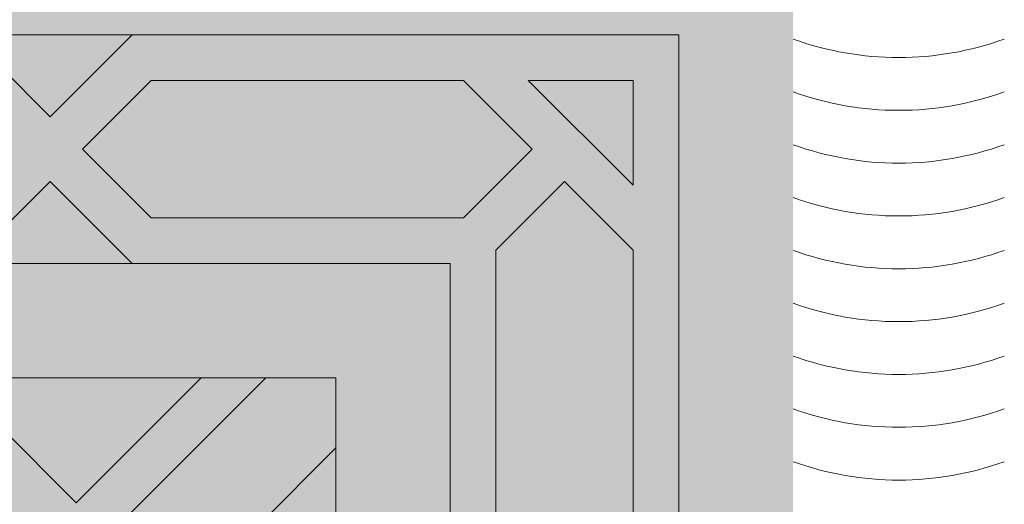
# Model space of a CAD drawing. Units: inches. Extents: x 844 to 2234, y 346 to 1084.
# Tile 39 of 93: x 1260.074 to 1265.567, y 705.079 to 707.782. Entities that reach past the tile are written whole.
import ezdxf

# ---------------------------------------------------------------- set-up
doc = ezdxf.new("R2010")
doc.units = ezdxf.units.IN
doc.header["$MEASUREMENT"] = 0
doc.layers.add('furniture', color=8, linetype='Continuous', lineweight=18)
doc.layers.add('RA-AP-01$0$INT', color=35, linetype='Continuous', lineweight=5)
doc.layers.add('RA-AP-01$0$FURN', color=3, linetype='Continuous')

# ---------------------------------------------------------------- blocks, each defined once
blk = doc.blocks.new('A$C18D01794')
at = {"layer": 'RA-AP-01$0$INT'}
h = blk.add_hatch(color=256, dxfattribs=at)
h.paths.add_polyline_path([(4.355206456958071, -6.156712009588037), (4.355206456958071, -8.056712009588038), (5.455206456958072, -8.056712009588038), (5.455206456958072, -6.156712009588037)])
h.paths.add_polyline_path([(4.405206456958072, -8.006712009588039), (4.405206456958072, -6.206712009588038), (5.405206456958072, -6.206712009588038), (5.405206456958072, -8.006712009588039)], flags=16)
h = blk.add_hatch(color=256, dxfattribs=at)
h.paths.add_polyline_path([(4.505206456958071, -7.585498806127123), (4.46934859260189, -7.549640941759413), (4.505206456958071, -7.513783077414768), (4.505206456958071, -7.381963272220687), (4.469348592616735, -7.346105407867824), (4.505206456958071, -7.310247543514964), (4.505206456958071, -7.178427738324996), (4.469348592586679, -7.142569873965138), (4.505206456952245, -7.106712009588038), (4.476922185709333, -7.106712009588038), (4.455206456960671, -7.128427738343681), (4.433490728198047, -7.106712009588038), (4.405206456946033, -7.106712009588036), (4.441064321339216, -7.142569873969684), (4.40520645695807, -7.178427738362358), (4.405206456958072, -7.310247543472698), (4.441064321364728, -7.346105407867826), (4.40520645695807, -7.381963272262947), (4.40520645695807, -7.513783077378263), (4.441064321354429, -7.549640941786153), (4.405206456958072, -7.585498806170974), (4.405206456958072, -7.717318611286652), (4.441064321333084, -7.753176475673194), (4.405206456958072, -7.789034340036673), (4.405206456958072, -8.006712009588039), (4.644348592588106, -8.006712009588039), (4.680206456964639, -7.970854145211967), (4.716064321341165, -8.006712009588039), (4.869348592586113, -8.006712009588039), (4.905206456964143, -7.970854145210465), (4.941064321342174, -8.006712009588039), (5.094348592587118, -8.006712009588037), (5.130206456963649, -7.970854145211967), (5.166064321340178, -8.006712009588039), (5.405206456958072, -8.006712009588039), (5.405206456958072, -7.789034340024526), (5.369348592595202, -7.753176475673196), (5.40520645695807, -7.717318611298797), (5.40520645695807, -7.585498806158829), (5.369348592573859, -7.549640941786151), (5.40520645695807, -7.51378307739041), (5.40520645695807, -7.381963272250803), (5.36934859256356, -7.346105407867824), (5.405206456958072, -7.310247543484846), (5.405206456958072, -7.178427738350217), (5.369348592589068, -7.142569873969682), (5.405206456982249, -7.106712009588038), (5.376922185730244, -7.106712009588038), (5.355206456967613, -7.128427738343679), (5.333490728218955, -7.10671200958804), (5.305206456976043, -7.106712009588042), (5.341064321341609, -7.142569873965136), (5.305206456958072, -7.178427738337141), (5.305206456958072, -7.310247543502816), (5.34106432131155, -7.346105407867824), (5.305206456958072, -7.381963272232832), (5.30520645695807, -7.513783077402624), (5.341064321326395, -7.549640941759413), (5.305206456958072, -7.585498806139263), (5.305206456958072, -7.717318611299605), (5.341064321347738, -7.753176475677737), (5.305206456958072, -7.78903434007894), (5.30520645695807, -7.906712009588039), (5.166064321336834, -7.906712009588039), (5.130206456963647, -7.942569873961684), (5.094348592590464, -7.906712009588039), (4.941064321338827, -7.906712009588041), (4.905206456964145, -7.942569873963183), (4.869348592589459, -7.906712009588039), (4.716064321337822, -7.906712009588041), (4.680206456964641, -7.942569873961684), (4.644348592591453, -7.906712009588039), (4.505206456958071, -7.906712009588039), (4.505206456958071, -7.789034340066795), (4.469348592580545, -7.753176475677738), (4.505206456958071, -7.717318611311748)])
h.paths.add_polyline_path([(4.485206456974132, -7.709034340046354), (4.45520645695909, -7.739034340051736), (4.425206456974128, -7.709034340057131), (4.425206456993394, -7.593783077384998), (4.45520645699153, -7.563783077396511), (4.485206456993396, -7.593783077408017)], flags=16)
h.paths.add_polyline_path([(4.455206456954537, -7.767318611299197), (4.485206456958242, -7.797318611312542), (4.48520645695951, -7.912569873958716), (4.45520645695415, -7.942569873954422), (4.425206456957888, -7.912569873967813), (4.425206456957888, -7.797318611286197)], flags=16)
h.paths.add_polyline_path([(4.455206456964794, -7.535498806149051), (4.42520645696469, -7.5054988061393), (4.425206456983954, -7.390247543486406), (4.455206456990734, -7.360247543489279), (4.485206456983953, -7.39024754349214), (4.485206456964687, -7.505498806158811)], flags=16)
h.paths.add_polyline_path([(4.499348592588947, -7.926712009585049), (4.636064321340932, -7.926712009585049), (4.666064321342317, -7.956712009586821), (4.636064321343707, -7.986712009585048), (4.499348592575121, -7.986712009585048), (4.469348592591685, -7.956712009591957)], flags=16)
h.paths.add_polyline_path([(4.425206456957888, -7.940854145195974), (4.471064321332215, -7.986712009585049), (4.425206456957888, -7.986712009585049)], flags=16)
h.paths.add_polyline_path([(4.455206456990734, -7.331963272246367), (4.425206456989053, -7.301963272254337), (4.425206456969784, -7.186712009596224), (4.455206456965226, -7.156712009591144), (4.485206456969787, -7.186712009586051), (4.485206456989053, -7.301963272238404)], flags=16)
h.paths.add_polyline_path([(4.72434859258714, -7.926712009586255), (4.861064321340141, -7.926712009586248), (4.891064321340324, -7.956712009586823), (4.861064321340513, -7.986712009586252), (4.724348592586768, -7.986712009586252), (4.694348592586956, -7.956712009586821)], flags=16)
h.paths.add_polyline_path([(4.919348592587961, -7.956712009586821), (4.949348592588145, -7.92671200958625), (5.08606432134115, -7.926712009586253), (5.116064321341327, -7.956712009586823), (5.086064321341519, -7.986712009586252), (4.949348592587774, -7.986712009586252)], flags=16)
h.paths.add_polyline_path([(5.144348592585967, -7.956712009586823), (5.174348592587358, -7.926712009585049), (5.311064321339338, -7.926712009585049), (5.3410643213366, -7.956712009591957), (5.311064321353163, -7.986712009585048), (5.174348592584576, -7.986712009585048)], flags=16)
h.paths.add_polyline_path([(5.32520645693489, -7.593783077408021), (5.355206456936755, -7.563783077396511), (5.385206456934894, -7.593783077384998), (5.38520645695416, -7.709034340057128), (5.355206456969194, -7.739034340051736), (5.325206456954153, -7.709034340046352)], flags=16)
h.paths.add_polyline_path([(5.325206456970042, -7.797318611312542), (5.355206456973747, -7.767318611299197), (5.385206456970398, -7.7973186112862), (5.385206456970398, -7.912569873967816), (5.355206456974136, -7.942569873954422), (5.325206456968778, -7.912569873958716)], flags=16)
h.paths.add_polyline_path([(5.325206456963599, -7.505498806158811), (5.325206456944333, -7.39024754349214), (5.355206456937552, -7.360247543489279), (5.385206456944332, -7.39024754348641), (5.385206456963596, -7.505498806139303), (5.355206456963492, -7.53549880614905)], flags=16)
h.paths.add_polyline_path([(5.32520645693923, -7.301963272238403), (5.3252064569585, -7.186712009586051), (5.355206456963062, -7.156712009591142), (5.3852064569585, -7.186712009596224), (5.385206456939234, -7.301963272254338), (5.355206456937552, -7.331963272246369)], flags=16)
h.paths.add_polyline_path([(5.339348592596071, -7.986712009585048), (5.385206456970398, -7.940854145195972), (5.385206456970396, -7.986712009585048)], flags=16)
h = blk.add_hatch(color=256, dxfattribs=at)
h.paths.add_polyline_path([(4.469348592586677, -7.142569873965136), (4.505206456958073, -7.178427738324996), (4.505206456958071, -7.106712009582215)])
h.paths.add_polyline_path([(4.455206456960671, -7.128427738343681), (4.476922185709333, -7.106712009588038), (4.433490728198045, -7.106712009588038)])
h.paths.add_polyline_path([(4.405206456958073, -7.178427738362358), (4.441064321339218, -7.142569873969684), (4.40520645695807, -7.106712009600073)])
h.paths.add_polyline_path([(4.425206456989053, -7.301963272254335), (4.455206456990736, -7.331963272246371), (4.485206456989055, -7.301963272238399), (4.48520645696979, -7.186712009586054), (4.455206456965227, -7.15671200959114), (4.425206456969784, -7.186712009596224)])
h.paths.add_polyline_path([(4.505206456958073, -7.381963272220689), (4.505206456958071, -7.310247543514961), (4.469348592616738, -7.346105407867826)])
h.paths.add_polyline_path([(4.425206456964688, -7.5054988061393), (4.455206456964794, -7.535498806149051), (4.485206456964689, -7.505498806158811), (4.485206456983951, -7.390247543492138), (4.455206456990736, -7.360247543489277), (4.425206456983956, -7.39024754348641)])
h.paths.add_polyline_path([(4.425206456974126, -7.709034340057128), (4.455206456959092, -7.739034340051736), (4.485206456974132, -7.709034340046356), (4.485206456993396, -7.593783077408017), (4.45520645699153, -7.563783077396511), (4.425206456993394, -7.593783077384999)])
h.paths.add_polyline_path([(4.46934859260189, -7.549640941759415), (4.505206456958071, -7.585498806127123), (4.505206456958073, -7.513783077414766)])
h.paths.add_polyline_path([(4.405206456958073, -7.585498806170972), (4.441064321354427, -7.549640941786151), (4.405206456958072, -7.513783077378263)])
h.paths.add_polyline_path([(4.405206456958072, -7.789034340036673), (4.441064321333084, -7.753176475673194), (4.405206456958072, -7.71731861128665)])
h.paths.add_polyline_path([(4.469348592580547, -7.75317647567774), (4.505206456958071, -7.789034340066795), (4.505206456958071, -7.717318611311744)])
h.paths.add_polyline_path([(4.425206456957888, -7.912569873967814), (4.45520645695415, -7.942569873954422), (4.485206456959507, -7.912569873958718), (4.48520645695824, -7.797318611312542), (4.455206456954537, -7.767318611299197), (4.425206456957888, -7.797318611286202)])
h.paths.add_polyline_path([(4.425206456957888, -7.986712009585049), (4.471064321332215, -7.986712009585049), (4.425206456957888, -7.940854145195972)])
h.paths.add_polyline_path([(4.499348592575121, -7.986712009585048), (4.636064321343707, -7.986712009585049), (4.666064321342317, -7.956712009586823), (4.636064321340932, -7.926712009585049), (4.499348592588945, -7.926712009585049), (4.469348592591685, -7.95671200959196)])
h.paths.add_polyline_path([(4.680206456964641, -7.942569873961684), (4.716064321337824, -7.906712009588039), (4.644348592591454, -7.906712009588039)])
h.paths.add_polyline_path([(4.644348592588108, -8.006712009588039), (4.716064321341167, -8.006712009588039), (4.680206456964637, -7.970854145211964)])
h.paths.add_polyline_path([(4.724348592586768, -7.98671200958625), (4.861064321340514, -7.986712009586252), (4.891064321340324, -7.956712009586819), (4.861064321340141, -7.92671200958625), (4.724348592587134, -7.926712009586255), (4.694348592586957, -7.956712009586821)])
h.paths.add_polyline_path([(4.905206456964143, -7.942569873963183), (4.941064321338827, -7.906712009588039), (4.869348592589457, -7.906712009588037)])
h.paths.add_polyline_path([(4.869348592586113, -8.006712009588039), (4.941064321342172, -8.006712009588037), (4.905206456964145, -7.970854145210463)])
h.paths.add_polyline_path([(4.949348592587774, -7.986712009586252), (5.086064321341521, -7.986712009586252), (5.116064321341329, -7.956712009586823), (5.08606432134115, -7.926712009586253), (4.949348592588145, -7.92671200958625), (4.919348592587961, -7.956712009586819)])
h.paths.add_polyline_path([(5.130206456963645, -7.942569873961684), (5.166064321336834, -7.906712009588039), (5.094348592590464, -7.906712009588039)])
h.paths.add_polyline_path([(5.094348592587119, -8.006712009588039), (5.166064321340178, -8.006712009588039), (5.130206456963651, -7.970854145211967)])
h.paths.add_polyline_path([(5.174348592584578, -7.986712009585048), (5.311064321353163, -7.986712009585048), (5.341064321336602, -7.956712009591958), (5.31106432133934, -7.926712009585049), (5.174348592587352, -7.926712009585049), (5.144348592585969, -7.956712009586823)])
h.paths.add_polyline_path([(5.325206456968778, -7.912569873958718), (5.355206456974136, -7.942569873954422), (5.385206456970396, -7.912569873967814), (5.385206456970396, -7.797318611286199), (5.355206456973747, -7.767318611299197), (5.325206456970044, -7.797318611312544)])
h.paths.add_polyline_path([(5.339348592596073, -7.986712009585048), (5.385206456970396, -7.986712009585049), (5.385206456970398, -7.94085414519597)])
h.paths.add_polyline_path([(5.325206456954155, -7.709034340046354), (5.355206456969194, -7.739034340051734), (5.38520645695416, -7.709034340057128), (5.385206456934896, -7.593783077384999), (5.355206456936758, -7.563783077396513), (5.325206456934888, -7.593783077408019)])
h.paths.add_polyline_path([(5.305206456958072, -7.789034340078938), (5.341064321347739, -7.753176475677738), (5.305206456958072, -7.717318611299605)])
h.paths.add_polyline_path([(5.369348592595204, -7.753176475673194), (5.40520645695807, -7.789034340024526), (5.405206456958072, -7.717318611298798)])
h.paths.add_polyline_path([(5.405206456958072, -7.585498806158831), (5.405206456958072, -7.513783077390407), (5.369348592573857, -7.549640941786151)])
h.paths.add_polyline_path([(5.305206456958072, -7.585498806139266), (5.341064321326393, -7.549640941759413), (5.305206456958072, -7.513783077402626)])
h.paths.add_polyline_path([(5.325206456963599, -7.50549880615881), (5.355206456963494, -7.535498806149055), (5.385206456963598, -7.505498806139302), (5.385206456944334, -7.390247543486411), (5.355206456937552, -7.360247543489279), (5.325206456944333, -7.39024754349214)])
h.paths.add_polyline_path([(5.305206456958072, -7.38196327223283), (5.341064321311551, -7.346105407867824), (5.305206456958072, -7.31024754350282)])
h.paths.add_polyline_path([(5.325206456939231, -7.301963272238404), (5.355206456937552, -7.331963272246369), (5.385206456939235, -7.301963272254335), (5.385206456958502, -7.186712009596224), (5.355206456963061, -7.156712009591142), (5.3252064569585, -7.186712009586051)])
h.paths.add_polyline_path([(5.404581768715993, -7.381338584008926, -0.001217816984214), (5.405206456958072, -7.381112009582329), (5.405206456958072, -7.310247543484846), (5.369348592563558, -7.346105407867826)])
h.paths.add_polyline_path([(5.36934859258907, -7.142569873969684), (5.40520645695807, -7.178427738350215), (5.405206456958072, -7.106712009612218)])
h.paths.add_polyline_path([(5.355206456967613, -7.128427738343683), (5.376922185730239, -7.106712009588038), (5.333490728218953, -7.10671200958804)])
h.paths.add_polyline_path([(5.30520645695807, -7.178427738337139), (5.341064321341609, -7.142569873965134), (5.305206456958074, -7.10671200957007)])
blk.add_hatch(color=256, dxfattribs=at).paths.add_polyline_path([(4.505206456958071, -7.906712009588039), (5.305206456958072, -7.906712009588039), (5.305206456958072, -7.106712009588038), (5.255206456951893, -7.106712009588036), (5.25520645694868, -7.856712009570104), (4.555206456959269, -7.856712009588616), (4.555206456956052, -7.106712009588038), (4.505206456958073, -7.106712009588038)])
h = blk.add_hatch(color=256, dxfattribs=at)
h.paths.add_polyline_path([(4.585917135068448, -7.856712009587804), (4.614201406330596, -7.856712009587056), (4.668846067270487, -7.802067348644738), (4.723490728212344, -7.856712009584164), (4.771774999457151, -7.856712009582887), (4.826419660396886, -7.80206734864072), (4.862780050090322, -7.838427738332541), (4.844495778842715, -7.856712009580965), (4.862780050090411, -7.856712009580482), (4.905206456960182, -7.814285602707865), (4.947632863832445, -7.856712009578238), (4.965917135079675, -7.856712009577755), (4.947632863831759, -7.838427738330656), (4.983993253523576, -7.802067348637219), (5.038637914464627, -7.856712009575829), (5.08692218571208, -7.856712009574554), (5.141566846649976, -7.802067348634224), (5.196211507589851, -7.856712009571666), (5.224495778822615, -7.856712009570916), (4.905206456953975, -7.537422687702283)])
h.paths.add_polyline_path([(4.895206456956031, -7.575706958950402), (4.895206456958921, -7.684996280828174), (4.840561796018589, -7.630351619890275)], flags=16)
h.paths.add_polyline_path([(4.915206456955638, -7.575706958949956), (4.969851117895509, -7.630351619887399), (4.915206456957609, -7.684996280827732)], flags=16)
h.paths.add_polyline_path([(4.826419660395175, -7.644493755514321), (4.881064321335613, -7.699138416452331), (4.771774999456703, -7.69913841645522)], flags=16)
h.paths.add_polyline_path([(4.983993253519558, -7.644493755510815), (5.038637914460456, -7.699138416449285), (4.929348592581548, -7.69913841645126)], flags=16)
h.paths.add_polyline_path([(4.881064321336025, -7.719138416452334), (4.826419660397532, -7.773783077393256), (4.771774999457062, -7.719138416455217)], flags=16)
h.paths.add_polyline_path([(4.929348592582019, -7.71913841645126), (5.038637914460982, -7.719138416449284), (4.983993253522945, -7.773783077389749)], flags=16)
h.paths.add_polyline_path([(4.895206456960191, -7.733280552075633), (4.895206456962115, -7.806001331460164), (4.876922185715016, -7.824285602708492), (4.840561796021581, -7.787925213016675)], flags=16)
h.paths.add_polyline_path([(4.915206456958487, -7.733280552075187), (4.969851117899527, -7.787925213013798), (4.933490728206909, -7.824285602708034), (4.9152064569598, -7.806001331461736)], flags=16)
h.paths.add_polyline_path([(4.757632863832376, -7.733280552079264), (4.812277524772842, -7.787925213017304), (4.757632863834348, -7.842569873958233)], flags=16)
h.paths.add_polyline_path([(4.737632863832376, -7.73328055207979), (4.737632863834348, -7.842569873958701), (4.682988202893906, -7.787925213020692)], flags=16)
h.paths.add_polyline_path([(5.05278005008503, -7.733280552072701), (5.052780050087917, -7.842569873951664), (4.998135389146995, -7.787925213013169)], flags=16)
h.paths.add_polyline_path([(5.072780050085024, -7.733280552072333), (5.127424711025931, -7.787925213010806), (5.072780050087916, -7.842569873951244)], flags=16)
h.paths.add_polyline_path([(4.935917135072783, -7.506712009583784), (5.255206456948811, -7.826001331459767), (5.255206456948932, -7.797717060211899), (5.200561796010279, -7.743072399273238), (5.255206456949403, -7.688427738334128), (5.25520645694961, -7.640143467086677), (5.200561796009787, -7.585498806146837), (5.236922185702417, -7.549138416454212), (5.255206456949919, -7.56742268770172), (5.255206456949998, -7.549138416454178), (5.212780050078687, -7.506712009583814), (5.25520645695036, -7.464285602712145), (5.255206456950438, -7.446001331464763), (5.236922185702424, -7.464285602712779), (5.200561796009796, -7.427925213020149), (5.255206456950753, -7.373280552079203), (5.25520645695096, -7.324996280834394), (5.200561796010322, -7.270351619893748), (5.255206456951428, -7.215706958952649), (5.255206456951547, -7.187422687705071)])
h.paths.add_polyline_path([(5.042988202883395, -7.42792521302065), (5.097632863823085, -7.373280552080975), (5.097632863822622, -7.482569873959883)], flags=16)
h.paths.add_polyline_path([(5.028846067259663, -7.442067348644384), (5.083490728198774, -7.496712009583504), (4.974201406321001, -7.496712009583035)], flags=16)
h.paths.add_polyline_path([(5.117632863823087, -7.37328055208089), (5.172277524762331, -7.42792521302015), (5.11763286382262, -7.482569873959851)], flags=16)
h.paths.add_polyline_path([(5.08349072819877, -7.516712009582191), (5.028846067259652, -7.571356670521302), (4.974201406320998, -7.516712009582638)], flags=16)
h.paths.add_polyline_path([(5.131774999446817, -7.35913841645716), (5.186419660386065, -7.413783077396415), (5.241064321325782, -7.359138416456712)], flags=17)
h.paths.add_polyline_path([(5.131774999446228, -7.496712009583703), (5.186419660386065, -7.442067348643883), (5.222780050079488, -7.478427738337313), (5.204495778832781, -7.496712009584014)], flags=16)
h.paths.add_polyline_path([(5.097632863822613, -7.530854145205813), (5.097632863823061, -7.640143467084723), (5.042988202883383, -7.585498806145032)], flags=16)
h.paths.add_polyline_path([(5.131774999446899, -7.339138416457162), (5.241064321325809, -7.339138416456712), (5.186419660386591, -7.284493755517479)], flags=17)
h.paths.add_polyline_path([(5.131774999446226, -7.516712009581999), (5.204495778830767, -7.516712009581702), (5.22278005007868, -7.534996280829206), (5.186419660386049, -7.571356670521828)], flags=16)
h.paths.add_polyline_path([(5.11763286382262, -7.530854145205852), (5.17227752476232, -7.585498806145562), (5.117632863823064, -7.64014346708481)], flags=16)
h.paths.add_polyline_path([(5.186419660386069, -7.599640941770585), (5.241064321325754, -7.654285602710281), (5.131774999446791, -7.654285602709814)], flags=16)
h.paths.add_polyline_path([(5.131774999446872, -7.674285602709813), (5.24106432132578, -7.674285602710282), (5.186419660386554, -7.728930263649504)], flags=16)
h.paths.add_polyline_path([(5.255206456951811, -7.126001331467467), (5.255206456951895, -7.106712009588038), (4.555206456956052, -7.106712009588038), (4.555206456956136, -7.12600133146746), (4.905206456953973, -7.476001331465289)])
h.paths.add_polyline_path([(4.983993253513404, -7.368930263651977), (4.92934859257295, -7.314285602713969), (5.03863791445186, -7.314285602711063)], flags=16)
h.paths.add_polyline_path([(4.969851117889988, -7.383072399276016), (4.915206456952556, -7.437717060215906), (4.915206456949648, -7.328427738338133)], flags=16)
h.paths.add_polyline_path([(4.929348592572535, -7.294285602713971), (4.983993253511019, -7.239640941773039), (5.038637914451496, -7.294285602711065)], flags=16)
h.paths.add_polyline_path([(5.052780050074912, -7.280143467087016), (4.998135389134438, -7.225498806148989), (5.052780050072919, -7.170854145208052)], flags=16)
h.paths.add_polyline_path([(5.07278005007491, -7.280143467086489), (5.072780050072918, -7.170854145207579), (5.127424711013374, -7.225498806145578)], flags=16)
h.paths.add_polyline_path([(4.89520645695295, -7.437717060216355), (4.840561796013067, -7.383072399278919), (4.895206456950961, -7.328427738338582)], flags=16)
h.paths.add_polyline_path([(4.915206456948365, -7.280143467090674), (4.915206456946434, -7.207422687704125), (4.933490728192729, -7.18913841645701), (4.969851117886972, -7.225498806149623)], flags=16)
h.paths.add_polyline_path([(4.881064321327021, -7.314285602715054), (4.82641966038902, -7.368930263655506), (4.771774999448108, -7.314285602717047)], flags=16)
h.paths.add_polyline_path([(4.895206456950073, -7.280143467091125), (4.840561796009022, -7.225498806152518), (4.876922185700835, -7.18913841645908), (4.895206456948749, -7.207422687706589)], flags=16)
h.paths.add_polyline_path([(4.983993253510392, -7.211356670525576), (4.947632863816944, -7.174996280833758), (4.965917135064043, -7.156712009585847), (5.038637914448995, -7.156712009584522)], flags=16)
h.paths.add_polyline_path([(4.881064321326543, -7.294285602715056), (4.771774999447578, -7.294285602717046), (4.826419660385607, -7.239640941776569)], flags=16)
h.paths.add_polyline_path([(4.905206456946447, -7.19913841645844), (4.862780050074785, -7.156712009587725), (4.947632863816685, -7.156712009586302)], flags=16)
h.paths.add_polyline_path([(5.14156684663679, -7.211356670521528), (5.086922185696452, -7.156712009583639), (5.196211507574223, -7.156712009581651)], flags=16)
h.paths.add_polyline_path([(4.8264196603837, -7.211356670529104), (4.771774999442643, -7.156712009590501), (4.8444957788276, -7.156712009588568), (4.862780050075511, -7.17499628083566)], flags=16)
h.paths.add_polyline_path([(4.812277524760289, -7.225498806153156), (4.757632863822258, -7.28014346709363), (4.757632863819352, -7.170854145214669)], flags=16)
h.paths.add_polyline_path([(4.73763286382226, -7.280143467093997), (4.682988202881349, -7.22549880615554), (4.737632863819352, -7.170854145215086)], flags=16)
h.paths.add_polyline_path([(4.723490728195188, -7.156712009591787), (4.668846067257299, -7.211356670532127), (4.614201406317417, -7.156712009594693)], flags=16)
h.paths.add_polyline_path([(4.597632863829262, -7.506712009583814), (4.555206456957951, -7.54913841645418), (4.555206456958029, -7.56742268770172), (4.573490728205535, -7.549138416454212), (4.609851117898167, -7.585498806146839), (4.555206456958338, -7.640143467086675), (4.555206456958546, -7.688427738334125), (4.60985111789767, -7.743072399273238), (4.555206456959015, -7.797717060211899), (4.555206456959138, -7.826001331459767), (4.874495778835167, -7.506712009583786), (4.5552064569564, -7.187422687705062), (4.555206456956523, -7.215706958952644), (4.609851117897629, -7.270351619893746), (4.555206456956988, -7.324996280834396), (4.555206456957198, -7.373280552079195), (4.609851117898153, -7.427925213020147), (4.573490728205528, -7.464285602712779), (4.555206456957507, -7.446001331464756), (4.555206456957585, -7.464285602712143)])
h.paths.add_polyline_path([(4.712780050085332, -7.482569873959882), (4.712780050084863, -7.373280552080972), (4.767424711024555, -7.42792521302065)], flags=16)
h.paths.add_polyline_path([(4.726922185709173, -7.496712009583504), (4.781566846648288, -7.442067348644384), (4.836211507586949, -7.496712009583033)], flags=16)
h.paths.add_polyline_path([(4.692780050085327, -7.482569873959851), (4.638135389145619, -7.427925213020149), (4.692780050084865, -7.373280552080892)], flags=16)
h.paths.add_polyline_path([(4.726922185709182, -7.516712009582191), (4.836211507586949, -7.51671200958264), (4.7815668466483, -7.571356670521304)], flags=16)
h.paths.add_polyline_path([(4.678637914461726, -7.496712009583706), (4.605917135075169, -7.496712009584014), (4.587632863828464, -7.478427738337311), (4.623993253521887, -7.442067348643881)], flags=16)
h.paths.add_polyline_path([(4.712780050085336, -7.530854145205816), (4.767424711024568, -7.585498806145034), (4.71278005008489, -7.640143467084724)], flags=16)
h.paths.add_polyline_path([(4.678637914461726, -7.516712009582001), (4.623993253521899, -7.571356670521829), (4.587632863829271, -7.534996280829206), (4.605917135077185, -7.5167120095817)], flags=16)
h.paths.add_polyline_path([(4.692780050085336, -7.530854145205848), (4.692780050084889, -7.64014346708481), (4.638135389145632, -7.585498806145562)], flags=16)
h.paths.add_polyline_path([(4.623993253521885, -7.413783077396415), (4.678637914461131, -7.359138416457161), (4.56934859258217, -7.359138416456712)], flags=17)
h.paths.add_polyline_path([(4.623993253521901, -7.599640941770568), (4.678637914461158, -7.654285602709814), (4.569348592582195, -7.654285602710281)], flags=16)
h.paths.add_polyline_path([(4.678637914461051, -7.339138416457162), (4.623993253521361, -7.284493755517479), (4.569348592582143, -7.339138416456712)], flags=17)
h.paths.add_polyline_path([(4.678637914461076, -7.674285602709813), (4.623993253521399, -7.728930263649504), (4.569348592582167, -7.674285602710281)], flags=16)
h = blk.add_hatch(color=256, dxfattribs=at)
h.paths.add_polyline_path([(4.905206456954232, -7.537422687702028), (4.874495778835232, -7.506712009583718), (4.555206456959138, -7.826001331459766), (4.555206456959269, -7.856712009588616), (4.585917135068449, -7.856712009587804)])
h.paths.add_polyline_path([(4.935917135072152, -7.506712009583152), (4.905206456953497, -7.537422687701806), (5.224495778822614, -7.856712009570917), (5.255206456948681, -7.856712009570104), (5.255206456948813, -7.826001331459768)])
h.paths.add_polyline_path([(5.255206456951549, -7.18742268770507), (5.255206456951813, -7.126001331467461), (4.905206456953563, -7.476001331465701), (4.935917135072559, -7.506712009584006)])
h.paths.add_polyline_path([(4.874495778835167, -7.506712009583785), (4.905206456953818, -7.476001331465132), (4.555206456956135, -7.126001331467458), (4.555206456956399, -7.187422687705064)])
h = blk.add_hatch(color=256, dxfattribs=at)
h.paths.add_polyline_path([(4.969851117891331, -7.630351619889621), (4.915206456952669, -7.575706958950966), (4.915206456952222, -7.684996280828739)])
h.paths.add_polyline_path([(4.895206456953064, -7.575706958950968), (4.840561796014413, -7.630351619889628), (4.895206456953533, -7.684996280828741)])
h.paths.add_polyline_path([(4.826419660390684, -7.644493755513362), (4.771774999451003, -7.699138416453052), (4.881064321329913, -7.699138416452587)])
h.paths.add_polyline_path([(4.881064321329884, -7.719138416452585), (4.771774999450921, -7.719138416453052), (4.82641966039018, -7.773783077392298)])
h.paths.add_polyline_path([(4.895206456953734, -7.733280552076196), (4.840561796013912, -7.787925213016031), (4.876922185707337, -7.824285602709455), (4.895206456954043, -7.806001331462747)])
h.paths.add_polyline_path([(4.862780050082808, -7.838427738332388), (4.826419660390178, -7.802067348639763), (4.771774999450351, -7.856712009579595), (4.844495778835303, -7.856712009579895)])
h.paths.add_polyline_path([(4.812277524766446, -7.787925213016036), (4.757632863827191, -7.733280552076788), (4.757632863826741, -7.842569873955747)])
h.paths.add_polyline_path([(4.737632863827191, -7.733280552076863), (4.682988202887508, -7.787925213016558), (4.737632863826743, -7.842569873955778)])
h.paths.add_polyline_path([(4.668846067263777, -7.802067348640287), (4.614201406325123, -7.856712009578949), (4.723490728202894, -7.856712009579402)])
h.paths.add_polyline_path([(4.905206456953846, -7.814285602708654), (4.862780050082654, -7.856712009579847), (4.947632863824561, -7.85671200958032)])
h.paths.add_polyline_path([(4.915206456952028, -7.733280552076195), (4.91520645695173, -7.806001331460731), (4.933490728199234, -7.824285602708648), (4.96985111789186, -7.787925213016022)])
h.paths.add_polyline_path([(5.038637914454841, -7.719138416453029), (4.929348592575874, -7.71913841645258), (4.983993253515593, -7.773783077392289)])
h.paths.add_polyline_path([(4.983993253515065, -7.644493755513352), (4.929348592575849, -7.699138416452582), (5.038637914454755, -7.699138416453031)])
h.paths.add_polyline_path([(5.052780050079843, -7.73328055207676), (4.998135389140595, -7.787925213016018), (5.052780050080309, -7.842569873955721)])
h.paths.add_polyline_path([(4.983993253516868, -7.802067348639752), (4.947632863824241, -7.838427738332383), (4.965917135071747, -7.856712009579888), (5.038637914456701, -7.856712009579572)])
h.paths.add_polyline_path([(5.127424711019533, -7.787925213016519), (5.072780050079843, -7.733280552076838), (5.07278005008031, -7.842569873955751)])
h.paths.add_polyline_path([(5.141566846643269, -7.802067348640248), (5.086922185704154, -7.85671200957937), (5.196211507581929, -7.856712009578901)])
for p, q in [((4.555206456956052, -7.106712009588036), (4.555206456959269, -7.856712009588616)), ((4.874495778835167, -7.506712009583786), (4.555206456959136, -7.826001331459769)), ((4.905206456953975, -7.537422687702283), (4.585917135071132, -7.856712009585121)), ((4.425206456957888, -7.797318611286199), (4.425206456957888, -7.912569873967814)), ((4.485206456959509, -7.912569873958718), (4.485206456958242, -7.797318611312544)), ((4.614201406333045, -7.85671200958461), (4.668846067270487, -7.802067348644737)), ((4.723490728210815, -7.856712009582635), (4.668846067270487, -7.802067348644737)), ((4.555206456959269, -7.856712009588616), (5.255206456948681, -7.856712009570104)), ((5.267206456961765, -7.906712009586254), (4.543206456966523, -7.906712009586254)), ((5.2672064569642, -7.906712009586255), (4.54320645696085, -7.906712009586255)), ((4.644348592589667, -7.906712009586254), (4.680206456964639, -7.942569873961684)), ((4.716064321339607, -7.906712009586254), (4.680206456964639, -7.942569873961684)), ((4.425206456957888, -7.912569873967814), (4.45520645695415, -7.942569873954422)), ((4.485206456959509, -7.912569873958718), (4.45520645695415, -7.942569873954422)), ((4.499348592588947, -7.926712009585049), (4.469348592591685, -7.956712009591957)), ((4.636064321340932, -7.926712009585049), (4.499348592588947, -7.926712009585049)), ((4.636064321340932, -7.926712009585049), (4.666064321342317, -7.956712009586823)), ((4.425206456957888, -7.940854145195974), (4.425206456957888, -7.986712009585049)), ((4.471064321332213, -7.986712009585048), (4.425206456957888, -7.940854145195974)), ((4.499348592575123, -7.986712009585048), (4.469348592591685, -7.956712009591957)), ((4.636064321343709, -7.986712009585049), (4.666064321342317, -7.956712009586823)), ((4.644348592589893, -8.006712009586252), (4.680206456964637, -7.970854145211966)), ((4.716064321339382, -8.006712009586252), (4.680206456964637, -7.970854145211966)), ((4.471064321332213, -7.986712009585048), (4.425206456957888, -7.986712009585049)), ((4.636064321343709, -7.986712009585049), (4.499348592575123, -7.986712009585048))]:
    blk.add_line(p, q, dxfattribs=at)
for points in [[(5.405206456958072, -8.006712009588039), (4.405206456958072, -8.006712009588039), (4.405206456958072, -7.106712009588038)], [(5.305206456958072, -7.106712009588038), (5.305206456958072, -7.906712009588039), (4.505206456958071, -7.906712009588039), (4.505206456958071, -7.106712009588038)]]:
    blk.add_lwpolyline(points, dxfattribs=at)
for centre in [(4.309006456952313, -7.948364458284338), (4.309006456952086, -7.971464458286042), (4.30900645694913, -7.994564458281608), (4.309006456948902, -8.017664458286497), (4.309006456951858, -8.040764458285018), (4.309006456950267, -8.063864458283767), (4.309006456948448, -8.086964458285472), (4.309006456948448, -8.11006445828422), (4.309006456946856, -8.13316445828297)]:
    blk.add_arc(centre, 0.136414042854523, 70.20384312815696, 109.7961568705686, dxfattribs=at)
blk = doc.blocks.new('A$C5D2F253E')
at = {"layer": 'RA-AP-01$0$FURN', "xscale": -0.7999999999883585, "yscale": 0.7999999999883585, "zscale": 0.8, "rotation": 90}
blk.add_blockref('A$C18D01794', (-5.687757199772477, 4.75791982714071), dxfattribs=at)

msp = doc.modelspace()

# ---------------------------------------------------------------- block references
at = {"layer": 'furniture', "xscale": -15.94108302203742, "yscale": 15.94108302203742, "zscale": 15.94108302203742, "rotation": 270}
msp.add_blockref('A$C5D2F253E', (1244.08405109492, 696.2584716700112), dxfattribs=at)

doc.saveas('drawing.dxf')
